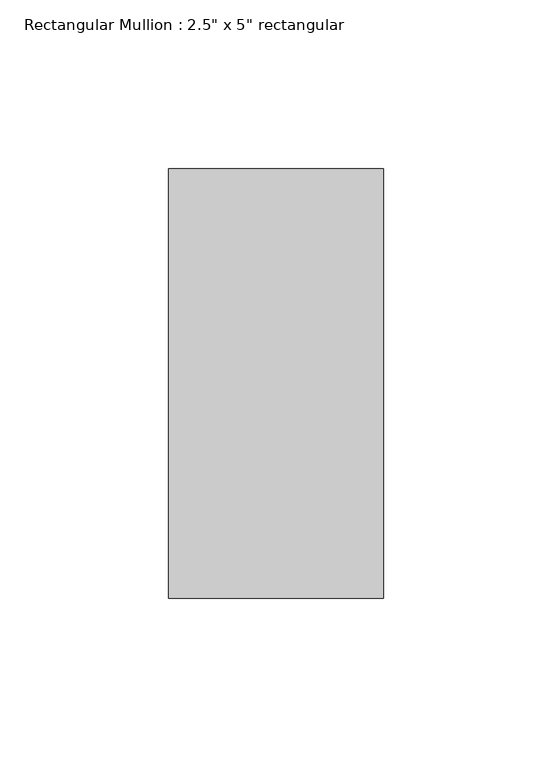
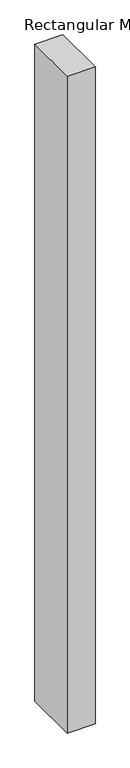
"""IFC4 building model written with IfcOpenShell, lengths in millimetres: member geometry."""

from ifc_helpers import new_model, si_unit, frame, origin, place, context, project, spatial, polyline, outline, extrude, source, transform, mapped, element, save


def member_43707fe5(model_context):
    return source(origin(), model_context, "Body", "SweptSolid", [
        extrude(outline(polyline([(31.75, 63.5), (31.75, -63.5), (-31.75, -63.5), (-31.75, 63.5), (31.75, 63.5)])), frame((0.0, 0.0, -1579.7129991), z_axis=(0.0, 0.0, 1.0), x_axis=(1.0, 0.0, 0.0)), (0.0, 0.0, 1.0), 1579.7129991),
    ])


if __name__ == "__main__":
    model = new_model("IFC4")
    model_context = context("Model", 3, world=origin())
    ifc_project = project(units=[si_unit("LENGTHUNIT", "METRE", prefix="MILLI")], contexts=[model_context])
    site = spatial("IfcSite", under=ifc_project)
    building = spatial("IfcBuilding", under=site)
    placement = place(None, origin())
    member_shape = member_43707fe5(model_context)
    element("IfcMember", 1, ObjectType="Rectangular Mullion : 2.5\" x 5\" rectangular", at=placement, inside=building, context=model_context, shape_type="MappedRepresentation", body=[
        mapped(member_shape, transform((0.0, 0.0, 0.0), x_axis=(1.0, 0.0, 0.0), y_axis=(0.0, 1.0, 0.0), z_axis=(0.0, 0.0, 1.0))),
    ])
    save(model, "model.ifc")

# Revit data of these elements
# Type "Rectangular Mullion : 2.5\" x 5\" rectangular"
#   built-in parameter 1007304 = 0.416667 (stored number, unit not read)
#   built-in parameter 1007301 = 0.104167 (stored number, unit not read)
#   built-in parameter 1007300 = 0.104167 (stored number, unit not read)
# Element 1 (IfcMember, "Rectangular Mullion : 2.5\" x 5\" rectangular")
#   Materials on its faces: "Aluminum"
# Materials
#   "Aluminum": class "Metal", colour RGB 247 247 247, transparency 0, Description = "Aluminum 6061", Cost = 0
